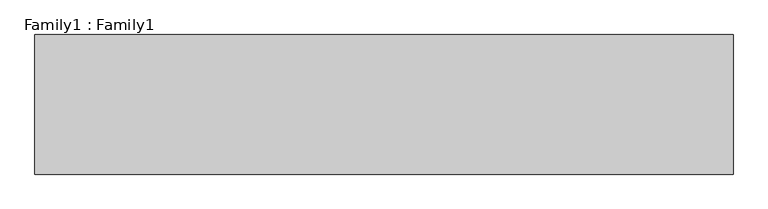
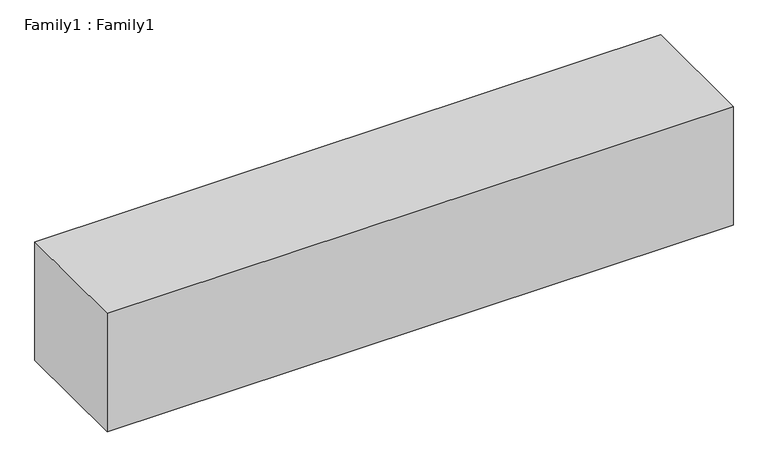
"""IFC4 building model written with IfcOpenShell, lengths in millimetres: furniture geometry, Family1 : Family1."""

from ifc_helpers import new_model, si_unit, origin, place, context, project, spatial, faceted_brep, source, transform, mapped, element, save


def family1_family1_08dda250(model_context):
    return source(origin(), model_context, "Body", "Brep", [
        faceted_brep([(762.0, 0.0, 304.8), (762.0, 304.8, 304.8), (-762.0, 304.8, 304.8), (-762.0, 0.0, 304.8), (762.0, 0.0, 0.0), (-762.0, 0.0, 0.0), (-762.0, 304.8, 0.0), (762.0, 304.8, 0.0), (711.2, 304.8, 254.0), (-711.2, 304.8, 254.0), (-711.2, 304.8, 50.8), (711.2, 304.8, 50.8), (711.2, 58.8837641, 254.0), (711.2, 58.8837641, 50.8), (-711.2, 58.8837641, 50.8), (-711.2, 58.8837641, 254.0)], [[[0, 1, 2, 3]], [[4, 5, 6, 7]], [[1, 0, 4, 7]], [[2, 1, 7, 6], [8, 9, 10, 11]], [[3, 2, 6, 5]], [[0, 3, 5, 4]], [[12, 13, 14, 15]], [[12, 15, 9, 8]], [[15, 14, 10, 9]], [[14, 13, 11, 10]], [[13, 12, 8, 11]]]),
    ])


if __name__ == "__main__":
    model = new_model("IFC4")
    model_context = context("Model", 3, world=origin())
    ifc_project = project(units=[si_unit("LENGTHUNIT", "METRE", prefix="MILLI")], contexts=[model_context])
    site = spatial("IfcSite", under=ifc_project)
    building = spatial("IfcBuilding", under=site)
    placement = place(None, origin())
    family1_family1_shape = family1_family1_08dda250(model_context)
    element("IfcFurniture", 1, ObjectType="Family1 : Family1", at=placement, inside=building, context=model_context, shape_type="MappedRepresentation", body=[
        mapped(family1_family1_shape, transform((0.0, 0.0, 0.0), x_axis=(1.0, 0.0, 0.0), y_axis=(0.0, 1.0, 0.0), z_axis=(0.0, 0.0, 1.0))),
    ])
    save(model, "model.ifc")

# Revit data of these elements
# Type "Family1 : Family1"
#   Default Elevation = 0
# Element 1 (IfcFurniture, "Family1 : Family1")
#   Materials on its faces: "wood"
# Materials
#   "wood": class "Generic", colour RGB 173 132 96, transparency 0, Cost = 0
